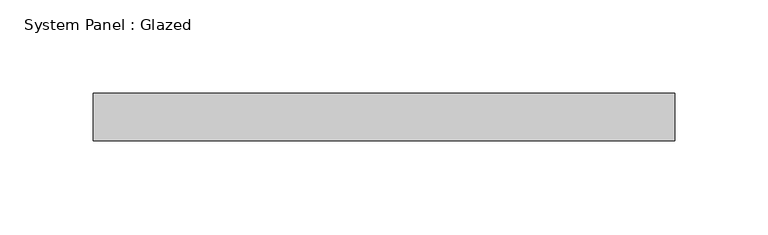
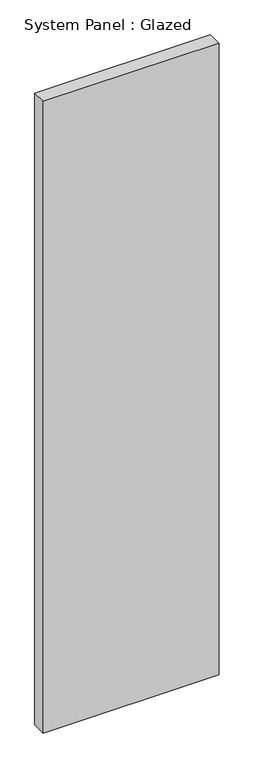
"""IFC4 building model written with IfcOpenShell, lengths in millimetres: plate geometry, System Panel : Glazed."""

from ifc_helpers import new_model, si_unit, origin, origin_with_axes, place, context, project, spatial, polyline, outline, extrude, source, transform, mapped, element, save


def system_panel_glazed_510f06c2(model_context):
    return source(origin(), model_context, "Body", "SweptSolid", [
        extrude(outline(polyline([(155.575, 19.05), (-155.575, 19.05), (-155.575, 44.45), (155.575, 44.45), (155.575, 19.05)])), origin_with_axes(), (0.0, 0.0, 1.0), 1181.1),
    ])


if __name__ == "__main__":
    model = new_model("IFC4")
    model_context = context("Model", 3, world=origin())
    ifc_project = project(units=[si_unit("LENGTHUNIT", "METRE", prefix="MILLI")], contexts=[model_context])
    site = spatial("IfcSite", under=ifc_project)
    building = spatial("IfcBuilding", under=site)
    placement = place(None, origin())
    system_panel_glazed_shape = system_panel_glazed_510f06c2(model_context)
    element("IfcPlate", 1, ObjectType="System Panel : Glazed", at=placement, inside=building, context=model_context, shape_type="MappedRepresentation", body=[
        mapped(system_panel_glazed_shape, transform((0.0, 0.0, 0.0), x_axis=(1.0, 0.0, 0.0), y_axis=(0.0, 1.0, 0.0), z_axis=(0.0, 0.0, 1.0))),
    ])
    save(model, "model.ifc")

# Revit data of these elements
# Type "System Panel : Glazed"
#   Construction Type Id = "GSP4R"
#   Analytic Construction = "1/8 in Pilkington single glazing"
#   Visual Light Transmittance = 0.9
#   Solar Heat Gain Coefficient = 0.86
#   Heat Transfer Coefficient (U) = 1.18115 BTU/(h·ft²·°F)
# Element 1 (IfcPlate, "System Panel : Glazed")
#   Materials on its faces: "Glass"
# Materials
#   "Glass": class "Glass", colour RGB 0 128 192, transparency 0.75, Description = "Soda Lime Glass", Cost = 0
